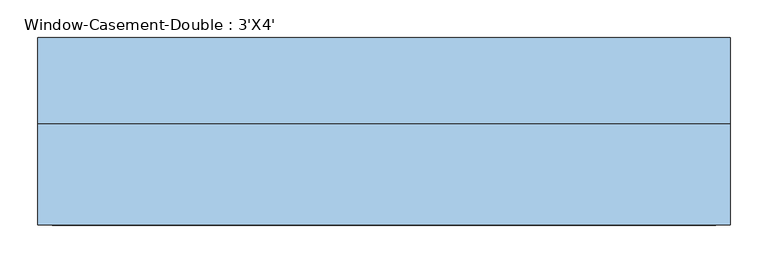
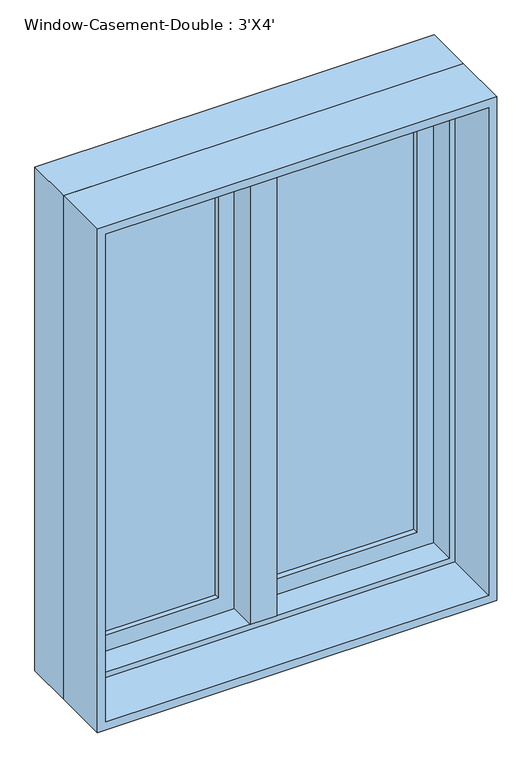
"""IFC4 building model written with IfcOpenShell, lengths in millimetres: window geometry, Window-Casement-Double : 3'X4'."""

from ifc_helpers import new_model, si_unit, frame, origin, place, context, project, spatial, polyline, outline, extrude, faceted_brep, source, transform, mapped, element, save


def window_casement_double_3_x4_d341e8ac(model_context):
    return source(origin(), model_context, "Body", "SolidModel", [
        faceted_brep([(9.525, 133.35, 2120.9), (-9.525, 133.35, 2120.9), (-9.525, 82.55, 2120.9), (9.525, 82.55, 2120.9), (9.525, 133.35, 927.1), (9.525, 82.55, 927.1), (-9.525, 82.55, 927.1), (-9.525, 133.35, 927.1), (-9.525, 82.55, 946.15), (-9.525, 82.55, 2101.85), (-30.1625, 82.55, 946.15), (-30.1625, 82.55, 2101.85), (-30.1625, 19.05, 946.15), (-30.1625, 19.05, 2101.85), (30.1625, 19.05, 946.15), (30.1625, 19.05, 2101.85), (30.1625, 82.55, 946.15), (30.1625, 82.55, 2101.85), (9.525, 82.55, 946.15), (9.525, 82.55, 2101.85)], [[[0, 1, 2, 3]], [[4, 5, 6, 7]], [[1, 0, 4, 7]], [[2, 1, 7, 6, 8, 9]], [[9, 8, 10, 11]], [[11, 10, 12, 13]], [[13, 12, 14, 15]], [[15, 14, 16, 17]], [[17, 16, 18, 19]], [[0, 3, 19, 18, 5, 4]], [[18, 8, 6, 5]], [[9, 19, 3, 2]], [[8, 18, 16, 14, 12, 10]], [[19, 9, 11, 13, 15, 17]]]),
        extrude(outline(polyline([(-66.675, 114.3), (-66.675, 107.95), (-387.35, 107.95), (-387.35, 114.3), (-66.675, 114.3)])), frame((0.0, 0.0, 984.25), z_axis=(0.0, 0.0, 1.0), x_axis=(1.0, 0.0, 0.0)), (0.0, 0.0, 1.0), 1079.5),
        extrude(outline(polyline([(-387.35, 95.25), (-387.35, 101.6), (-66.675, 101.6), (-66.675, 95.25), (-387.35, 95.25)])), frame((0.0, 0.0, 984.25), z_axis=(0.0, 0.0, 1.0), x_axis=(1.0, 0.0, 0.0)), (0.0, 0.0, 1.0), 1079.5),
        extrude(outline(polyline([(387.35, 114.3), (387.35, 107.95), (66.675, 107.95), (66.675, 114.3), (387.35, 114.3)])), frame((0.0, 0.0, 984.25), z_axis=(0.0, 0.0, 1.0), x_axis=(1.0, 0.0, 0.0)), (0.0, 0.0, 1.0), 1079.5),
        extrude(outline(polyline([(66.675, 95.25), (66.675, 101.6), (387.35, 101.6), (387.35, 95.25), (66.675, 95.25)])), frame((0.0, 0.0, 984.25), z_axis=(0.0, 0.0, 1.0), x_axis=(1.0, 0.0, 0.0)), (0.0, 0.0, 1.0), 1079.5),
        extrude(outline(polyline([(2120.9, -444.5), (927.1, -444.5), (927.1, -9.525), (2120.9, -9.525), (2120.9, -444.5)]), holes=[polyline([(2063.75, -66.675), (984.25, -66.675), (984.25, -387.35), (2063.75, -387.35), (2063.75, -66.675)])]), frame((0.0, 82.55, 0.0), z_axis=(0.0, 1.0, 0.0), x_axis=(0.0, 0.0, 1.0)), (0.0, 0.0, 1.0), 44.45),
        extrude(outline(polyline([(927.1, 444.5), (2120.9, 444.5), (2120.9, 9.525), (927.1, 9.525), (927.1, 444.5)]), holes=[polyline([(984.25, 66.675), (2063.75, 66.675), (2063.75, 387.35), (984.25, 387.35), (984.25, 66.675)])]), frame((0.0, 82.55, 0.0), z_axis=(0.0, 1.0, 0.0), x_axis=(0.0, 0.0, 1.0)), (0.0, 0.0, 1.0), 44.45),
        extrude(outline(polyline([(2133.6, -457.2), (914.4, -457.2), (914.4, 457.2), (2133.6, 457.2), (2133.6, -457.2)]), holes=[polyline([(2114.55, 438.15), (933.45, 438.15), (933.45, -438.15), (2114.55, -438.15), (2114.55, 438.15)])]), frame((0.0, -114.3, 0.0), z_axis=(0.0, 1.0, 0.0), x_axis=(0.0, 0.0, 1.0)), (0.0, 0.0, 1.0), 133.35),
        faceted_brep([(425.45, 82.55, 2101.85), (425.45, 19.05, 2101.85), (-425.45, 19.05, 2101.85), (-425.45, 82.55, 2101.85), (444.5, 133.35, 2120.9), (444.5, 82.55, 2120.9), (-444.5, 82.55, 2120.9), (-444.5, 133.35, 2120.9), (457.2, 19.05, 2133.6), (457.2, 133.35, 2133.6), (-457.2, 133.35, 2133.6), (-457.2, 19.05, 2133.6), (-425.45, 19.05, 946.15), (-425.45, 82.55, 946.15), (-444.5, 82.55, 927.1), (-444.5, 133.35, 927.1), (-457.2, 133.35, 914.4), (-457.2, 19.05, 914.4), (425.45, 19.05, 946.15), (425.45, 82.55, 946.15), (444.5, 82.55, 927.1), (444.5, 133.35, 927.1), (457.2, 133.35, 914.4), (457.2, 19.05, 914.4)], [[[0, 1, 2, 3]], [[4, 5, 6, 7]], [[8, 9, 10, 11]], [[3, 2, 12, 13]], [[7, 6, 14, 15]], [[11, 10, 16, 17]], [[13, 12, 18, 19]], [[15, 14, 20, 21]], [[17, 16, 22, 23]], [[11, 17, 23, 8], [1, 18, 12, 2]], [[19, 18, 1, 0]], [[5, 20, 14, 6], [3, 13, 19, 0]], [[21, 20, 5, 4]], [[23, 22, 9, 8]], [[9, 22, 16, 10], [7, 15, 21, 4]]]),
    ])


if __name__ == "__main__":
    model = new_model("IFC4")
    model_context = context("Model", 3, world=origin())
    ifc_project = project(units=[si_unit("LENGTHUNIT", "METRE", prefix="MILLI")], contexts=[model_context])
    site = spatial("IfcSite", under=ifc_project)
    building = spatial("IfcBuilding", under=site)
    placement = place(None, origin())
    window_casement_double_3_x4_shape = window_casement_double_3_x4_d341e8ac(model_context)
    element("IfcWindow", 1, ObjectType="Window-Casement-Double : 3'X4'", at=placement, inside=building, context=model_context, shape_type="MappedRepresentation", body=[
        mapped(window_casement_double_3_x4_shape, transform((0.0, 0.0, 0.0), x_axis=(1.0, 0.0, 0.0), y_axis=(0.0, 1.0, 0.0), z_axis=(0.0, 0.0, 1.0))),
    ])
    save(model, "model.ifc")

# Revit data of these elements
# Type "Window-Casement-Double : 3'X4'"
#   Type Mark = "21"
#   Fire Rating = "0.5h"
#   Assembly Code = "B2020100"
#   Analytic Construction = "Double glazing - domestic"
#   Frame Extension [instance default] = 0' - 0 1/4"
#   Window Inset [instance default] = 0' - 0"
#   Wall Thickness [instance default] = 0' - 6"
#   Interior Wall Closure [instance default] = 0' - 2 1/4"
#   Half Width = 1' - 6"
#   Visual Light Transmittance = 0.81
#   Thermal Resistance (R) = 1.8146 (h·ft²·°F)/BTU
#   Solar Heat Gain Coefficient = 0.76
#   Rough Width = 3' - 0 1/2"
#   Rough Height = 4' - 0 1/2"
#   Height = 4' - 0"
#   Heat Transfer Coefficient (U) = 0.5511 BTU/(h·ft²·°F)
#   Exterior Wall Closure [instance default] = 0' - 1 1/4"
#   Extension Jamb [instance default] = 0' - 2 1/4"
#   Default Sill Height = 3' - 0"
#   Width = 3' - 0"
#   Muntin Visibility = yes
#   Interior Trim Visibility [instance default] = yes
#   Exterior Trim Visibility [instance default] = yes
#   Extension Jamb Visibility [instance default] = yes
#   Interior Trim Material = Wood - Stained
#   Muntin Pattern = Muntin Pattern_2x2 : Muntin Pattern_2x2
#   Interior Trim = Trim-Window-Interior-Flat : Picture Frame
#   Interior Frame Material = Wood - Stained
#   Glass Panel Material = Glass
#   Exterior Trim Material = Clad - White
#   Exterior Trim = Trim-Window-Exterior-Flat : with Sill
#   Exterior Frame Material = Clad - White
#   Wall Closure = (empty or 0)
# Element 1 (IfcWindow, "Window-Casement-Double : 3'X4'")
#   Wall Thickness = 0' - 9"
#   Extension Jamb = 0' - 5 1/4"
#   Materials on its faces: "Wood - Stained", "Glass", "Clad - White"
# Materials
#   "Wood - Stained": class "Wood", colour RGB 224 178 126, transparency 0, Cost = 0
#   "Glass": class "Glass", colour RGB 0 128 192, transparency 0.75, Description = "Soda Lime Glass", Cost = 0
#   "Clad - White": class "Wood", colour RGB 242 242 238, transparency 0, Cost = 0
